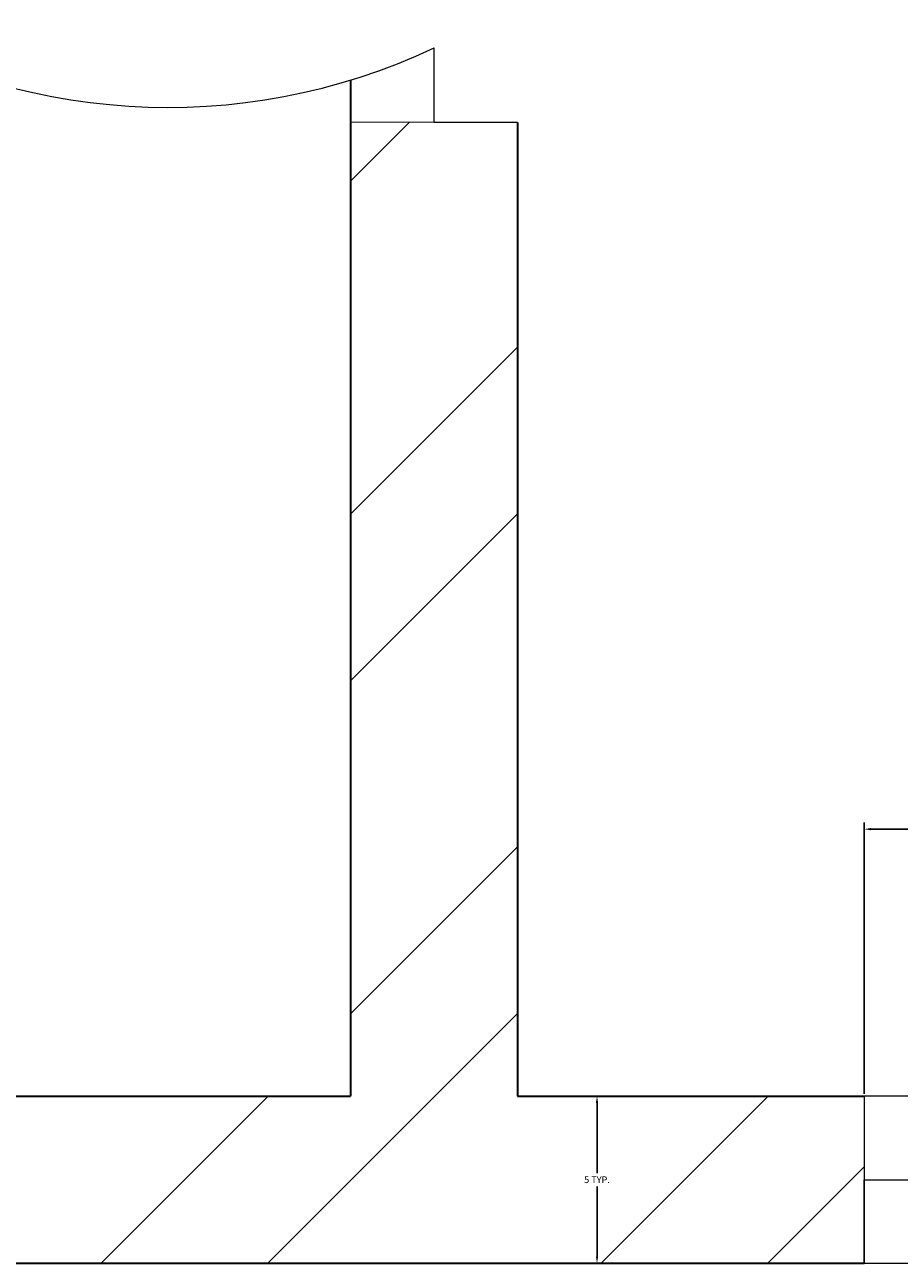
# Model space of a CAD drawing. Units: inches. Extents: x 1885 to 2748, y 783 to 2421.
# Tile 44 of 117: x 2216 to 2240, y 1558 to 1591. Entities that reach past the tile are written whole.
import ezdxf

# ---------------------------------------------------------------- set-up
doc = ezdxf.new("R2010")
doc.units = ezdxf.units.IN
for name, color, linetype, lineweight in [('A-ANNO-DIMS', 2, 'Continuous', 18), ('A-DOOR', 31, 'Continuous', 18), ('A-GLAZ', 181, 'Continuous', 18), ('A-WALL', 7, 'Continuous', 35)]:
    doc.layers.add(name, color=color, linetype=linetype, lineweight=lineweight)
doc.layers.add('A-WALL-PATT', color=85, linetype='Continuous', lineweight=13, true_color=0x58ba48)
doc.styles.get("Standard").update_dxf_attribs({"font": 'arial.ttf'})
doc.dimstyles.get("Standard").update_dxf_attribs({"dimtxt": 0.18, "dimasz": 0.18, "dimexe": 0.18, "dimexo": 0.0625, "dimgap": 0.09, "dimtad": 0, "dimtih": 1, "dimtoh": 1, "dimdec": 4, "dimzin": 0, "dimdsep": 46, "dimtxsty": 'Standard', "dimcen": 0.09, "dimadec": 0, "dimazin": 0, "dimtfac": 1, "dimtdec": 4, "dimtofl": 0, "dimtmove": 0, "dimatfit": 3, "dimfxl": 1, "dimtolj": 1, "dimtzin": 0, "dimarcsym": 0})

# ---------------------------------------------------------------- blocks, each defined once
blk = doc.blocks.new('WIN-48')
for p, q in [((0.003, 4.496), (0.003, -0.004)), ((48.003, 4.496), (0.003, 4.496)), ((0.003, -0.004), (0.003, 2.246)), ((0.003, 2.246), (48.003, 2.246)), ((0.003, -0.004), (48.003, -0.004))]:
    blk.add_line(p, q)
blk = doc.blocks.new('*D25')
at = {"layer": 'A-ANNO-DIMS', "color": 0, "lineweight": -2, "transparency": 16777216}
for p, q in [((2238.613, 1562.568), (2238.613, 1569.886)), ((2238.793, 1569.706), (2261.495, 1569.706)), ((2286.433, 1569.706), (2263.732, 1569.706)), ((2286.613, 1562.568), (2286.613, 1569.886))]:
    blk.add_line(p, q, dxfattribs=at)
at = {"layer": 'A-ANNO-DIMS', "color": 0, "transparency": 16777216}
for points in [[(2238.793, 1569.736), (2238.793, 1569.676), (2238.613, 1569.706)], [(2286.433, 1569.736), (2286.433, 1569.676), (2286.613, 1569.706)]]:
    blk.add_solid(points, dxfattribs=at)
at = {"layer": 'Defpoints', "color": 0, "transparency": 16777216}
for p in [(2286.613, 1569.706), (2238.613, 1562.506), (2286.613, 1562.506)]:
    blk.add_point(p, dxfattribs=at)
at = {"layer": 'A-ANNO-DIMS', "color": 0, "transparency": 16777216, "insert": (2262.613, 1569.706), "char_height": 0.18, "attachment_point": 5}
blk.add_mtext('\\A1;WINDOW 48 TYP.', dxfattribs=at)
blk = doc.blocks.new('*D26')
at = {"layer": 'A-ANNO-DIMS', "color": 0, "lineweight": -2, "transparency": 16777216}
for p, q in [((2238.551, 1562.506), (2231.233, 1562.506)), ((2231.413, 1562.326), (2231.413, 1560.437)), ((2231.413, 1558.186), (2231.413, 1560.074)), ((2238.551, 1558.006), (2231.233, 1558.006))]:
    blk.add_line(p, q, dxfattribs=at)
at = {"layer": 'A-ANNO-DIMS', "color": 0, "transparency": 16777216}
for points in [[(2231.383, 1562.326), (2231.443, 1562.326), (2231.413, 1562.506)], [(2231.383, 1558.186), (2231.443, 1558.186), (2231.413, 1558.006)]]:
    blk.add_solid(points, dxfattribs=at)
at = {"layer": 'Defpoints', "color": 0, "transparency": 16777216}
for p in [(2231.413, 1562.506), (2238.613, 1562.506), (2238.613, 1558.006)]:
    blk.add_point(p, dxfattribs=at)
at = {"layer": 'A-ANNO-DIMS', "color": 0, "transparency": 16777216, "insert": (2231.413, 1560.256), "char_height": 0.18, "attachment_point": 5}
blk.add_mtext('\\A1;5 TYP.', dxfattribs=at)

msp = doc.modelspace()

# ---------------------------------------------------------------- hatches: boundary and pattern name
at = {"layer": 'A-WALL-PATT'}
h = msp.add_hatch(dxfattribs=at)
h.set_pattern_fill('ANSI32', color=256)
h.paths.add_polyline_path([(2007.772, 2318.006), (1980.774, 2318.006), (1980.774, 2281.215), (1985.274, 2281.215), (1985.274, 2313.506), (2007.772, 2313.506), (2007.772, 2315.756)])
h.paths.add_polyline_path([(2094.324, 2318.006), (2067.772, 2318.006), (2067.772, 2313.506), (2094.324, 2313.506), (2094.324, 2315.756)])
h.paths.add_polyline_path([(2131.367, 2315.756), (2131.367, 2318.006), (2131.189, 2318.006), (2112.609, 2318.006), (2112.609, 2313.506), (2117.274, 2313.506), (2117.274, 2255.201), (2121.774, 2255.201), (2121.774, 2313.506), (2131.367, 2313.506)])
h.paths.add_polyline_path([(2190.512, 2318.006), (2155.367, 2318.006), (2155.367, 2313.506), (2169.774, 2313.506), (2169.774, 2229.506), (2121.774, 2229.506), (2121.774, 2233.451), (2119.524, 2233.451), (2117.274, 2233.451), (2117.274, 2201.101), (2121.774, 2201.101), (2121.774, 2225.006), (2169.774, 2225.006), (2169.774, 2165.006), (2306.274, 2165.006), (2306.274, 2066.006), (2310.774, 2066.006), (2344.274, 2066.006), (2486.274, 2066.006), (2486.274, 1886.006), (2483.02, 1886.006), (2483.02, 1881.506), (2486.274, 1881.506), (2486.274, 1880.678), (2490.774, 1880.678), (2490.774, 2070.506), (2344.274, 2070.506), (2310.774, 2070.506), (2310.774, 2165.006), (2310.774, 2173.636), (2308.524, 2173.636), (2306.274, 2173.636), (2306.274, 2169.506), (2174.274, 2169.506), (2174.274, 2313.506), (2190.512, 2313.506), (2190.512, 2315.756)])
h.paths.add_polyline_path([(1985.274, 2221.215), (1980.774, 2221.215), (1980.774, 2165.006), (1992.774, 2165.006), (1992.774, 2141.927), (1997.274, 2141.927), (1997.274, 2165.006), (2117.274, 2165.006), (2117.274, 2163.126), (2121.774, 2163.126), (2121.774, 2172.734), (2119.524, 2172.734), (2117.274, 2172.734), (2117.274, 2169.506), (1985.274, 2169.506)])
h.paths.add_polyline_path([(1997.274, 2105.927), (1992.774, 2105.927), (1992.774, 2070.506), (2016.774, 2070.506), (2016.774, 2059.123), (2019.024, 2059.123), (2021.274, 2059.123), (2021.274, 2070.506), (2117.274, 2070.506), (2117.274, 2022.506), (2114.423, 2022.506), (2114.423, 2018.006), (2123.627, 2018.006), (2123.627, 2020.256), (2123.627, 2022.506), (2121.774, 2022.506), (2121.774, 2142.587), (2119.524, 2142.587), (2117.274, 2142.587), (2117.274, 2075.006), (1997.274, 2075.006)])
h.paths.add_polyline_path([(2092.029, 2020.256), (2092.029, 2022.506), (2021.274, 2022.506), (2021.274, 2035.123), (2016.774, 2035.123), (2016.774, 2018.006), (2016.774, 1978.784), (2021.274, 1978.784), (2021.274, 2018.006), (2092.029, 2018.006)])
h.paths.add_polyline_path([(2260.938, 2022.506), (2153.105, 2022.506), (2153.105, 2020.256), (2153.105, 2018.006), (2155.274, 2018.006), (2155.274, 1886.006), (2107.629, 1886.006), (2107.629, 1881.506), (2182.911, 1881.506), (2182.911, 1883.756), (2182.911, 1886.006), (2159.774, 1886.006), (2159.774, 2018.006), (2260.938, 2018.006), (2260.938, 2020.256)])
h.paths.add_polyline_path([(2047.629, 1883.756), (2047.629, 1886.006), (2021.274, 1886.006), (2021.274, 1918.784), (2019.024, 1918.784), (2016.774, 1918.784), (2016.774, 1881.506), (2047.629, 1881.506)])
h.paths.add_polyline_path([(2306.361, 1883.756), (2306.361, 1886.006), (2296.274, 1886.006), (2296.274, 1982.006), (2316.535, 1982.006), (2316.535, 1984.256), (2316.535, 1986.506), (2296.274, 1986.506), (2296.274, 2022.506), (2289.276, 2022.506), (2289.276, 2018.006), (2291.774, 2018.006), (2291.774, 1886.006), (2242.911, 1886.006), (2242.911, 1881.506), (2306.361, 1881.506)], flags=17)
h.paths.add_polyline_path([(1985.274, 1843.006), (2021.6, 1843.006), (2021.534, 1845.441), (2021.477, 1847.506), (1980.774, 1847.506), (1980.774, 1809.446), (1985.274, 1809.446)])
h.paths.add_polyline_path([(2131.482, 1845.256), (2131.482, 1847.506), (2081.534, 1847.506), (2081.534, 1843.006), (2117.274, 1843.006), (2117.274, 1784.147), (2119.524, 1784.147), (2121.774, 1784.147), (2121.774, 1843.006), (2131.482, 1843.006)])
h.paths.add_polyline_path([(2203.886, 1847.506), (2155.482, 1847.506), (2155.482, 1843.006), (2169.774, 1843.006), (2169.774, 1759.006), (2121.774, 1759.006), (2121.774, 1761.457), (2117.274, 1761.457), (2117.274, 1730.429), (2121.774, 1730.429), (2121.774, 1754.506), (2177.421, 1754.506), (2177.421, 1756.756), (2177.421, 1759.006), (2174.274, 1759.006), (2174.274, 1843.006), (2203.886, 1843.006)])
h.paths.add_polyline_path([(2335.554, 1845.256), (2335.554, 1847.506), (2239.886, 1847.506), (2239.886, 1843.006), (2306.274, 1843.006), (2306.274, 1759.006), (2199.486, 1759.006), (2199.486, 1754.506), (2310.774, 1754.506), (2310.774, 1843.006), (2335.554, 1843.006)])
h.paths.add_polyline_path([(2348.774, 2022.506), (2344.274, 2022.506), (2344.274, 1986.506), (2341.681, 1986.506), (2341.681, 1982.006), (2344.274, 1982.006), (2344.274, 1886.006), (2330.361, 1886.006), (2330.361, 1881.506), (2361.627, 1881.506), (2361.627, 1883.756), (2361.627, 1886.006), (2348.774, 1886.006)], flags=17)
h.paths.add_polyline_path([(2283.251, 2315.756), (2283.251, 2318.006), (2238.512, 2318.006), (2238.512, 2313.506), (2283.251, 2313.506)], flags=17)
h.paths.add_polyline_path([(2363.274, 2348.006), (2388.677, 2348.006), (2388.677, 2350.256), (2388.677, 2352.506), (2358.774, 2352.506), (2358.774, 2348.006), (2358.774, 2318.006), (2344.481, 2318.006), (2344.481, 2313.506), (2358.774, 2313.506), (2358.774, 2229.506), (2310.774, 2229.506), (2310.774, 2231.952), (2306.274, 2231.952), (2306.274, 2205.611), (2310.774, 2205.611), (2310.774, 2225.006), (2358.774, 2225.006), (2358.774, 2211.506), (2452.329, 2211.506), (2452.329, 2213.756), (2452.329, 2216.006), (2363.274, 2216.006), (2363.274, 2318.006)])
h.paths.add_polyline_path([(2310.774, 2313.506), (2320.481, 2313.506), (2320.481, 2315.756), (2320.481, 2318.006), (2302.728, 2318.006), (2302.728, 2313.506), (2306.274, 2313.506), (2306.274, 2251.076), (2310.774, 2251.076)], flags=17)
h.paths.add_polyline_path([(2490.774, 2352.506), (2486.274, 2352.506), (2448.677, 2352.506), (2448.677, 2348.006), (2486.274, 2348.006), (2486.274, 2318.006), (2486.274, 2216.006), (2481.78, 2216.006), (2481.78, 2211.506), (2486.274, 2211.506), (2486.274, 2165.006), (2493.289, 2165.006), (2493.289, 2167.256), (2493.289, 2169.506), (2490.774, 2169.506), (2490.774, 2313.506), (2494.429, 2313.506), (2494.429, 2318.006), (2490.774, 2318.006)])
h.paths.add_polyline_path([(2534.653, 2318.006), (2515.691, 2318.006), (2515.691, 2313.506), (2534.653, 2313.506), (2534.653, 2315.756)])
h.paths.add_polyline_path([(2618.274, 2318.006), (2594.653, 2318.006), (2594.653, 2313.506), (2613.774, 2313.506), (2613.774, 2281.706), (2618.274, 2281.706)])
h.paths.add_polyline_path([(2618.274, 2221.706), (2613.774, 2221.706), (2613.774, 2169.506), (2554.019, 2169.506), (2554.019, 2165.006), (2613.774, 2165.006), (2613.774, 2152.878), (2618.274, 2152.878)])
h.paths.add_polyline_path([(2618.274, 2128.878), (2616.024, 2128.878), (2613.774, 2128.878), (2613.774, 2117.006), (2529.774, 2117.006), (2529.774, 2165.006), (2532.848, 2165.006), (2532.848, 2169.506), (2522.867, 2169.506), (2522.867, 2165.006), (2525.274, 2165.006), (2525.274, 2117.006), (2525.274, 2112.506), (2525.274, 2108.576), (2529.774, 2108.576), (2529.774, 2112.506), (2613.774, 2112.506), (2613.774, 2080.19), (2618.274, 2080.19)])
h.paths.add_polyline_path([(2618.274, 2044.19), (2616.024, 2044.19), (2613.774, 2044.19), (2613.774, 2015.506), (2529.774, 2015.506), (2529.774, 2088.582), (2527.524, 2088.582), (2525.274, 2088.582), (2525.274, 2011.006), (2613.774, 2011.006), (2613.774, 1956.755), (2618.274, 1956.755)])
h.paths.add_polyline_path([(2618.274, 1881.506), (2618.274, 1896.755), (2613.774, 1896.755), (2613.774, 1881.506), (2613.774, 1847.506), (2592.715, 1847.506), (2592.715, 1843.006), (2613.774, 1843.006), (2613.774, 1765.006), (2613.774, 1760.506), (2609.621, 1760.506), (2609.621, 1756.006), (2613.774, 1756.006), (2613.774, 1660.006), (2608.544, 1660.006), (2608.544, 1655.506), (2613.774, 1655.506), (2613.774, 1508.158), (2618.274, 1508.158)])
h.paths.add_polyline_path([(2565.774, 1843.006), (2568.997, 1843.006), (2568.997, 1847.506), (2490.774, 1847.506), (2490.774, 1849.7), (2488.524, 1849.7), (2486.274, 1849.7), (2486.274, 1847.506), (2477.274, 1847.506), (2477.274, 1838.506), (2477.274, 1821.493), (2486.274, 1821.493), (2486.274, 1838.506), (2561.274, 1838.506), (2561.274, 1765.006), (2486.274, 1765.006), (2486.274, 1786.157), (2477.274, 1786.157), (2477.274, 1765.006), (2477.274, 1756.006), (2486.274, 1756.006), (2565.774, 1756.006), (2585.621, 1756.006), (2585.621, 1758.256), (2585.621, 1760.506), (2565.774, 1760.506), (2565.774, 1765.006)])
h.paths.add_polyline_path([(2486.274, 1651.006), (2561.274, 1651.006), (2561.274, 1567.006), (2486.274, 1567.006), (2486.274, 1591.321), (2477.274, 1591.321), (2477.274, 1567.006), (2477.274, 1558.006), (2477.274, 1555.439), (2481.774, 1555.439), (2481.774, 1558.006), (2568.653, 1558.006), (2568.653, 1560.256), (2568.653, 1562.506), (2565.774, 1562.506), (2565.774, 1655.506), (2584.544, 1655.506), (2584.544, 1657.756), (2584.544, 1660.006), (2565.774, 1660.006), (2486.274, 1660.006), (2477.274, 1660.006), (2477.274, 1651.006), (2477.274, 1632.989), (2486.274, 1632.989)])
h.paths.add_polyline_path([(2449.967, 1883.756), (2449.967, 1886.006), (2421.627, 1886.006), (2421.627, 1881.506), (2449.967, 1881.506)], flags=17)
h.paths.add_polyline_path([(2447.274, 1847.506), (2395.554, 1847.506), (2395.554, 1843.006), (2442.774, 1843.006), (2442.774, 1809.27), (2447.274, 1809.27)])
h.paths.add_polyline_path([(1985.274, 1749.446), (1980.774, 1749.446), (1980.774, 1694.504), (1985.274, 1694.504), (1985.274, 1694.506), (1986.897, 1694.506), (1986.897, 1697.78), (1986.897, 1699.006), (1985.274, 1699.006)])
h.paths.add_polyline_path([(2152.774, 1699.006), (2121.774, 1699.006), (2121.774, 1703.668), (2119.524, 1703.668), (2117.274, 1703.668), (2117.274, 1699.006), (2009.219, 1699.006), (2009.219, 1694.506), (2148.274, 1694.506), (2148.274, 1692.631), (2152.774, 1692.631)])
h.paths.add_polyline_path([(2016.274, 1694.506), (2011.774, 1694.506), (2011.774, 1558.006), (2040.806, 1558.006), (2040.806, 1560.256), (2040.806, 1562.506), (2016.274, 1562.506)])
h.paths.add_polyline_path([(2152.774, 1663.017), (2150.524, 1663.017), (2148.274, 1663.017), (2148.274, 1562.506), (2100.806, 1562.506), (2100.806, 1558.006), (2165.119, 1558.006), (2165.119, 1560.256), (2165.119, 1562.506), (2152.774, 1562.506), (2152.774, 1610.506), (2224.774, 1610.506), (2224.774, 1607.99), (2229.274, 1607.99), (2229.274, 1615.006), (2152.774, 1615.006)])
h.paths.add_polyline_path([(2238.613, 1560.256), (2238.613, 1562.506), (2229.274, 1562.506), (2229.274, 1588.756), (2227.024, 1588.763), (2224.774, 1588.771), (2224.774, 1562.506), (2189.119, 1562.506), (2189.119, 1558.006), (2238.613, 1558.006)])
h.paths.add_polyline_path([(2336.024, 1560.256), (2336.024, 1562.506), (2310.774, 1562.506), (2310.774, 1656.347), (2308.524, 1656.347), (2306.274, 1656.347), (2306.274, 1562.506), (2286.613, 1562.506), (2286.613, 1558.006), (2336.024, 1558.006)])
h.paths.add_polyline_path([(2447.274, 1690.968), (2445.024, 1690.968), (2442.774, 1690.968), (2442.774, 1687.006), (2306.274, 1687.006), (2306.274, 1680.75), (2310.774, 1680.75), (2310.774, 1682.506), (2442.774, 1682.506), (2442.774, 1562.506), (2396.024, 1562.506), (2396.024, 1558.006), (2447.274, 1558.006)])
h.paths.add_polyline_path([(2447.274, 1749.27), (2445.024, 1749.27), (2442.774, 1749.27), (2442.774, 1717.232), (2447.274, 1717.232)])
h.paths.add_polyline_path([(2044.674, 1521.756), (2044.674, 1524.006), (2007.274, 1524.006), (2007.274, 1503.49), (2009.524, 1503.49), (2011.774, 1503.49), (2011.774, 1519.506), (2044.674, 1519.506)])
h.paths.add_polyline_path([(2177.969, 1521.756), (2177.969, 1524.006), (2104.674, 1524.006), (2104.674, 1519.506), (2145.774, 1519.506), (2145.774, 1387.506), (2143.37, 1387.506), (2143.37, 1383.006), (2251.585, 1383.006), (2251.585, 1385.256), (2251.585, 1387.506), (2150.274, 1387.506), (2150.274, 1519.506), (2177.969, 1519.506)])
h.paths.add_polyline_path([(2298.704, 1524.006), (2237.969, 1524.006), (2237.969, 1519.506), (2282.274, 1519.506), (2282.274, 1387.506), (2279.683, 1387.506), (2279.683, 1383.006), (2286.774, 1383.006), (2286.774, 1419.006), (2312.451, 1419.006), (2312.451, 1421.256), (2312.451, 1423.506), (2286.774, 1423.506), (2286.774, 1519.506), (2298.704, 1519.506), (2298.704, 1521.722)], flags=17)
h.paths.add_polyline_path([(2361.897, 1521.756), (2361.897, 1524.006), (2322.704, 1524.006), (2322.704, 1519.506), (2334.774, 1519.506), (2334.774, 1423.506), (2331.93, 1423.506), (2331.93, 1419.006), (2334.774, 1419.006), (2334.774, 1387.506), (2334.774, 1383.228), (2339.274, 1383.228), (2339.274, 1387.506), (2339.274, 1519.506), (2361.897, 1519.506)], flags=17)
h.paths.add_polyline_path([(2447.274, 1521.756), (2447.274, 1524.006), (2421.897, 1524.006), (2421.897, 1519.506), (2447.274, 1519.506)], flags=17)
h.paths.add_polyline_path([(2481.774, 1529.6), (2479.524, 1529.6), (2477.274, 1529.6), (2477.274, 1524.006), (2474.489, 1524.006), (2474.489, 1519.506), (2477.274, 1519.506), (2477.274, 1334.506), (2296.774, 1334.506), (2296.774, 1240.506), (2160.274, 1240.506), (2160.274, 1180.506), (2112.274, 1180.506), (2112.274, 1207.692), (2110.024, 1207.692), (2107.774, 1207.692), (2107.774, 1171.609), (2112.274, 1171.609), (2112.274, 1176.006), (2160.274, 1176.006), (2160.274, 1092.006), (2144.221, 1092.006), (2144.221, 1087.506), (2189.497, 1087.506), (2189.497, 1089.756), (2189.497, 1092.006), (2164.774, 1092.006), (2164.774, 1236.006), (2296.774, 1236.006), (2296.774, 1231.912), (2301.274, 1231.912), (2301.274, 1330.006), (2481.774, 1330.006), (2481.774, 1387.506)])
h.paths.add_polyline_path([(2618.274, 1448.158), (2613.774, 1448.158), (2613.774, 1382.506), (2529.774, 1382.506), (2525.274, 1382.506), (2525.274, 1307.062), (2529.774, 1307.062), (2529.774, 1378.006), (2613.774, 1378.006), (2613.774, 1354.988), (2618.274, 1354.988)])
h.paths.add_polyline_path([(2618.274, 1318.988), (2613.774, 1318.988), (2613.774, 1281.006), (2529.774, 1281.006), (2529.774, 1283.786), (2527.524, 1283.786), (2525.274, 1283.786), (2525.274, 1228.506), (2516.794, 1228.506), (2516.794, 1224.006), (2533.484, 1224.006), (2533.484, 1226.256), (2533.484, 1228.506), (2529.774, 1228.506), (2529.774, 1276.506), (2613.774, 1276.506), (2613.774, 1266.02), (2618.274, 1266.02)])
h.paths.add_polyline_path([(2618.274, 1134.964), (2613.774, 1134.964), (2613.774, 1092.006), (2594.545, 1092.006), (2594.545, 1087.506), (2618.274, 1087.506)])
h.paths.add_polyline_path([(2534.545, 1092.006), (2509.765, 1092.006), (2509.765, 1087.506), (2534.545, 1087.506), (2534.545, 1089.756)])
h.paths.add_polyline_path([(2481.274, 1224.006), (2484.117, 1224.006), (2484.117, 1226.256), (2484.117, 1228.506), (2476.774, 1228.506), (2476.774, 1198.506), (2471.61, 1198.506), (2471.61, 1194.006), (2476.774, 1194.006), (2476.774, 1062.006), (2436.894, 1062.006), (2436.894, 1057.506), (2476.774, 1057.506), (2481.274, 1057.506), (2481.274, 1062.006), (2481.274, 1087.506), (2485.354, 1087.506), (2485.354, 1089.756), (2485.354, 1092.006), (2481.274, 1092.006), (2481.274, 1117.506)])
h.paths.add_polyline_path([(2439.898, 1198.506), (2349.274, 1198.506), (2349.274, 1194.006), (2349.274, 1180.506), (2301.274, 1180.506), (2301.274, 1201.896), (2299.024, 1201.896), (2296.774, 1201.896), (2296.774, 1172.335), (2299.024, 1172.335), (2301.274, 1172.335), (2301.274, 1176.006), (2349.274, 1176.006), (2349.274, 1092.006), (2334.452, 1092.006), (2334.452, 1087.506), (2349.274, 1087.506), (2349.274, 1057.506), (2353.774, 1057.506), (2376.894, 1057.506), (2376.894, 1059.756), (2376.894, 1062.006), (2353.774, 1062.006), (2353.774, 1087.506), (2353.774, 1180.506), (2353.774, 1194.006), (2439.898, 1194.006), (2439.898, 1196.256)])
h.paths.add_polyline_path([(2270.596, 1089.756), (2270.596, 1092.006), (2249.497, 1092.006), (2249.497, 1087.506), (2270.596, 1087.506)], flags=17)
h.paths.add_polyline_path([(2310.452, 1092.006), (2301.274, 1092.006), (2301.274, 1153.292), (2296.774, 1153.292), (2296.774, 1092.006), (2293.786, 1092.006), (2293.786, 1087.506), (2310.452, 1087.506), (2310.452, 1089.756)], flags=17)
h.paths.add_polyline_path([(2112.274, 1150.328), (2110.024, 1150.328), (2107.774, 1150.328), (2107.774, 1092.006), (2104.465, 1092.006), (2104.465, 1087.506), (2120.221, 1087.506), (2120.221, 1089.756), (2120.221, 1092.006), (2112.274, 1092.006)])
h.paths.add_polyline_path([(2082.172, 1092.006), (2058.144, 1092.006), (2058.144, 1087.506), (2082.172, 1087.506), (2082.172, 1089.756)])
h.paths.add_polyline_path([(1975.774, 1145.638), (1971.274, 1145.638), (1971.274, 1087.506), (1980.774, 1087.506), (1998.144, 1087.506), (1998.144, 1089.756), (1998.144, 1092.006), (1985.274, 1092.006), (1975.774, 1092.006)])
h.paths.add_polyline_path([(2112.274, 1244.385), (2110.024, 1244.385), (2107.774, 1244.385), (2107.774, 1240.506), (1992.274, 1240.506), (1992.274, 1271.008), (1987.774, 1271.008), (1987.774, 1240.506), (1980.774, 1240.506), (1975.774, 1240.506), (1971.274, 1240.506), (1971.274, 1205.638), (1975.774, 1205.638), (1975.774, 1236.006), (2107.774, 1236.006), (2107.774, 1233.444), (2112.274, 1233.444), (2112.274, 1236.006)])
h.paths.add_polyline_path([(2112.274, 1383.006), (2114.783, 1383.006), (2114.783, 1385.256), (2114.783, 1387.506), (2102.476, 1387.506), (2102.476, 1383.006), (2107.774, 1383.006), (2107.774, 1335.006), (2011.774, 1335.006), (2011.774, 1349.939), (2007.274, 1349.939), (2007.274, 1335.006), (1987.774, 1335.006), (1987.774, 1330.506), (1987.774, 1307.008), (1992.274, 1307.008), (1992.274, 1330.506), (2007.274, 1330.506), (2107.774, 1330.506), (2107.774, 1264.711), (2112.274, 1264.711)])
h.paths.add_polyline_path([(2077.857, 1387.506), (2011.774, 1387.506), (2011.774, 1390.036), (2009.524, 1390.036), (2007.274, 1390.036), (2007.274, 1373.939), (2011.774, 1373.939), (2011.774, 1383.006), (2077.857, 1383.006)])
h.paths.add_polyline_path([(2011.774, 1443.49), (2007.274, 1443.49), (2007.274, 1410.248), (2011.774, 1410.248)])

# ---------------------------------------------------------------- linework, layer by layer
at = {"layer": 'A-DOOR'}
for p, q in [((2227.024, 1588.763), (2227.024, 1590.763)), ((2224.774, 1588.771), (2229.274, 1588.756)), ((2229.274, 1588.756), (2227.024, 1588.763))]:
    msp.add_line(p, q, dxfattribs=at)
msp.add_arc((2219.854, 1605.99), 16.83, 180, 295.2133, dxfattribs=at)
at = {"layer": 'A-WALL'}
for p, q in [((2224.774, 1589.895), (2224.774, 1562.506)), ((2229.274, 1588.756), (2229.274, 1562.506)), ((2189.119, 1562.506), (2224.774, 1562.506)), ((2229.274, 1562.506), (2238.613, 1562.506)), ((2189.119, 1558.006), (2238.613, 1558.006))]:
    msp.add_line(p, q, dxfattribs=at)

# ---------------------------------------------------------------- block references
at = {"layer": 'A-GLAZ'}
msp.add_blockref('WIN-48', (2238.61, 1558.01), dxfattribs=at)

# ---------------------------------------------------------------- dimensions: what is measured, and where the dimension line sits
at = {"layer": 'A-ANNO-DIMS'}
dim = msp.add_linear_dim(base=(2286.613, 1569.706), p1=(2238.613, 1562.506), p2=(2286.613, 1562.506), text='WINDOW <> TYP.', dimstyle='Standard', override={"dimdec": 0, "dimlfac": 1, "dimrnd": 0, "dimzin": 0, "dimdsep": 46, "dimlunit": 2}, dxfattribs=at)
dim.commit()
dim.dimension.update_dxf_attribs({"geometry": '*D25', "text_midpoint": (2262.613, 1569.706)})
dim = msp.add_linear_dim(base=(2231.413161565, 1562.505556822), p1=(2238.613161565, 1558.005556822), p2=(2238.613161565, 1562.505556822), angle=90, text='<> TYP.', dimstyle='Standard', override={"dimdec": 0, "dimlfac": 1, "dimrnd": 0, "dimzin": 0, "dimdsep": 46, "dimlunit": 2}, dxfattribs=at)
dim.commit()
dim.dimension.update_dxf_attribs({"geometry": '*D26', "text_midpoint": (2231.413161565, 1560.255556822)})

doc.saveas('drawing.dxf')
